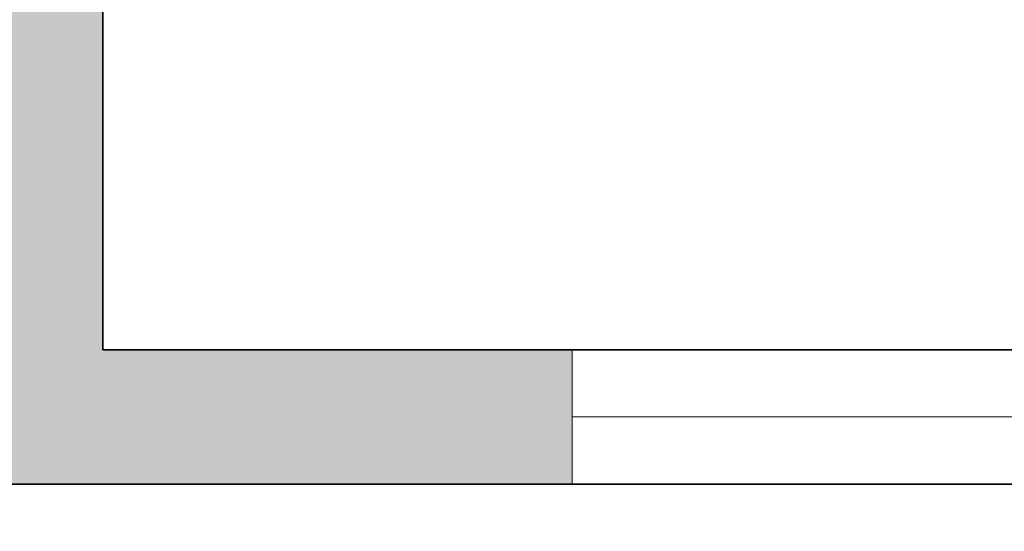
# Model space of a CAD drawing. Units: inches. Extents: x 1319 to 2030, y 219 to 1069.
# Tile 18 of 28: x 1433 to 1499, y 549 to 583. Entities that reach past the tile are written whole.
import ezdxf

# ---------------------------------------------------------------- set-up
doc = ezdxf.new("R2010")
doc.units = ezdxf.units.IN
doc.header["$MEASUREMENT"] = 0
for name, color, linetype, lineweight in [('A-GLAZ', 4, 'Continuous', 18), ('A-WALL-PATT', 252, 'Continuous', 13), ('walls', 250, 'Continuous', 35)]:
    doc.layers.add(name, color=color, linetype=linetype, lineweight=lineweight)

msp = doc.modelspace()

# ---------------------------------------------------------------- hatches: boundary and pattern name
at = {"layer": 'A-WALL-PATT'}
h = msp.add_hatch(color=256, dxfattribs=at)
h.dxf.hatch_style = 1
h.paths.add_polyline_path([(1856.292, 860.616), (1812.343, 860.616), (1812.343, 851.616), (1812.343, 700.993), (1816.843, 700.993), (1816.843, 851.616), (1856.292, 851.616)])
h.paths.add_polyline_path([(1960.843, 663.616), (1812.343, 663.616), (1782.783, 663.616), (1782.783, 659.116), (1812.343, 659.116), (1960.843, 659.116)])
h.paths.add_polyline_path([(1857.424, 659.116), (1852.924, 659.116), (1852.924, 616.807), (1857.424, 616.807)])
h.paths.add_polyline_path([(1735.843, 661.727), (1731.843, 661.727), (1636.133, 661.727), (1636.133, 657.227), (1731.343, 657.227), (1731.343, 481.227), (1618.616, 481.227), (1618.616, 472.227), (1639.343, 472.227), (1639.343, 384.227), (1627.044, 384.227), (1627.044, 375.227), (1648.343, 375.227), (1648.343, 384.227), (1648.343, 472.227), (1750.706, 472.227), (1750.706, 481.227), (1735.843, 481.227), (1735.843, 657.727)])
h.paths.add_polyline_path([(1587.343, 481.227), (1578.343, 481.227), (1578.343, 375.227), (1597.622, 375.227), (1597.622, 384.227), (1587.343, 384.227)])
h.paths.add_polyline_path([(1769.593, 384.227), (1693.482, 384.227), (1693.482, 375.227), (1769.593, 375.227)])
h.paths.add_polyline_path([(1775.828, 481.227), (1765.831, 481.227), (1765.831, 472.227), (1775.828, 472.227)])
h.paths.add_polyline_path([(1824.625, 481.227), (1820.343, 481.227), (1820.343, 476.727), (1824.625, 476.727), (1824.625, 477.545)], flags=0)
h.paths.add_polyline_path([(1896.843, 481.227), (1852.26, 481.227), (1852.26, 476.727), (1892.343, 476.727), (1892.343, 384.227), (1881.742, 384.227), (1881.742, 375.227), (1913.435, 375.227), (1913.435, 384.227), (1896.843, 384.227)])
h.paths.add_polyline_path([(1960.843, 481.227), (1931.341, 481.227), (1931.341, 476.727), (1960.843, 476.727)])
h.paths.add_polyline_path([(1736.343, 918.227), (1731.843, 918.227), (1731.843, 890.227), (1582.843, 890.227), (1582.843, 781.727), (1582.843, 769.171), (1587.343, 769.171), (1587.343, 781.727), (1587.343, 885.727), (1731.843, 885.727), (1731.843, 851.616), (1736.343, 851.616), (1736.343, 890.227)])
h.paths.add_polyline_path([(1781.022, 860.616), (1773.021, 860.616, -0.032228), (1773.289, 856.464), (1773.289, 851.616), (1781.022, 851.616)])
h.paths.add_polyline_path([(1587.343, 946.227), (1582.843, 946.227), (1582.843, 926.136), (1587.343, 926.136)])
h.paths.add_polyline_path([(1647.843, 946.227), (1643.343, 946.227), (1643.343, 926.136), (1647.843, 926.136)])
h.paths.add_polyline_path([(1543.343, 786.227), (1429.843, 786.227), (1429.843, 757.555), (1434.343, 757.555), (1438.843, 757.555), (1438.843, 781.727), (1543.343, 781.727)])
h.paths.add_polyline_path([(1543.343, 781.727), (1538.843, 781.727), (1538.843, 709.727), (1534.597, 709.727), (1534.597, 705.227), (1543.343, 705.227), (1543.343, 709.727)])
h.paths.add_polyline_path([(1499.955, 709.727), (1438.843, 709.727), (1438.843, 734.463), (1429.843, 734.463), (1429.843, 552.227), (1470.241, 552.227), (1470.241, 561.227), (1438.843, 561.227), (1438.843, 705.227), (1499.955, 705.227)])
h.paths.add_polyline_path([(1587.343, 709.727), (1582.843, 709.727), (1582.843, 561.227), (1543.433, 561.227), (1543.433, 552.227), (1587.343, 552.227)])
h.paths.add_polyline_path([(1546.835, 709.727), (1543.343, 709.727), (1543.343, 705.227), (1546.835, 705.227)])
h.paths.add_polyline_path([(1582.843, 709.727), (1579.15, 709.727), (1579.15, 705.227), (1582.843, 705.227)], flags=17)
h.paths.add_polyline_path([(1548.368, 786.227), (1543.343, 786.227), (1543.343, 781.727), (1548.368, 781.727)])
h.paths.add_polyline_path([(1582.843, 786.227), (1580.683, 786.227), (1580.683, 781.727), (1582.843, 781.727)])
h.paths.add_polyline_path([(1587.343, 892.402), (1582.843, 892.402), (1582.843, 890.227), (1587.343, 890.227)], flags=17)
h.paths.add_polyline_path([(1647.843, 892.402), (1643.343, 892.402), (1643.343, 890.227), (1647.843, 890.227)], flags=17)
h.paths.add_polyline_path([(1740.974, 856.464), (1740.974, 860.616), (1736.343, 860.616), (1736.343, 851.616), (1740.974, 851.616)])
h.paths.add_polyline_path([(1853.989, 384.227), (1820.343, 384.227), (1820.343, 402.924), (1815.843, 402.924), (1815.843, 375.227), (1853.989, 375.227)])
h.paths.add_polyline_path([(1892.343, 436.227), (1820.343, 436.227), (1820.343, 481.227), (1815.843, 481.227), (1815.843, 431.727), (1892.343, 431.727)])
h.paths.add_polyline_path([(1849.175, 481.227), (1824.625, 481.227), (1824.625, 477.545), (1825.699, 477.545), (1825.699, 453.018, 0.401453), (1849.175, 477.545)], flags=0)
h.paths.add_polyline_path([(1960.843, 384.227), (1941.188, 384.227), (1941.188, 375.227), (1960.843, 375.227)])
h.paths.add_polyline_path([(1902.267, 481.227), (1896.843, 481.227), (1896.843, 476.727), (1902.267, 476.727), (1902.267, 477.44)], flags=0)

# ---------------------------------------------------------------- linework, layer by layer
at = {"layer": 'A-GLAZ'}
for p, q in [((1470.241, 561.227), (1470.241, 552.227)), ((1543.433, 561.227), (1470.241, 561.227)), ((1470.241, 561.227), (1470.241, 556.727)), ((1470.241, 556.727), (1543.433, 556.727)), ((1470.241, 552.227), (1543.433, 552.227))]:
    msp.add_line(p, q, dxfattribs=at)
at = {"layer": 'walls'}
for p, q in [((1438.843, 561.227), (1438.843, 705.227)), ((1438.843, 561.227), (1582.843, 561.227)), ((1429.843, 552.227), (1587.343, 552.227))]:
    msp.add_line(p, q, dxfattribs=at)

doc.saveas('drawing.dxf')
